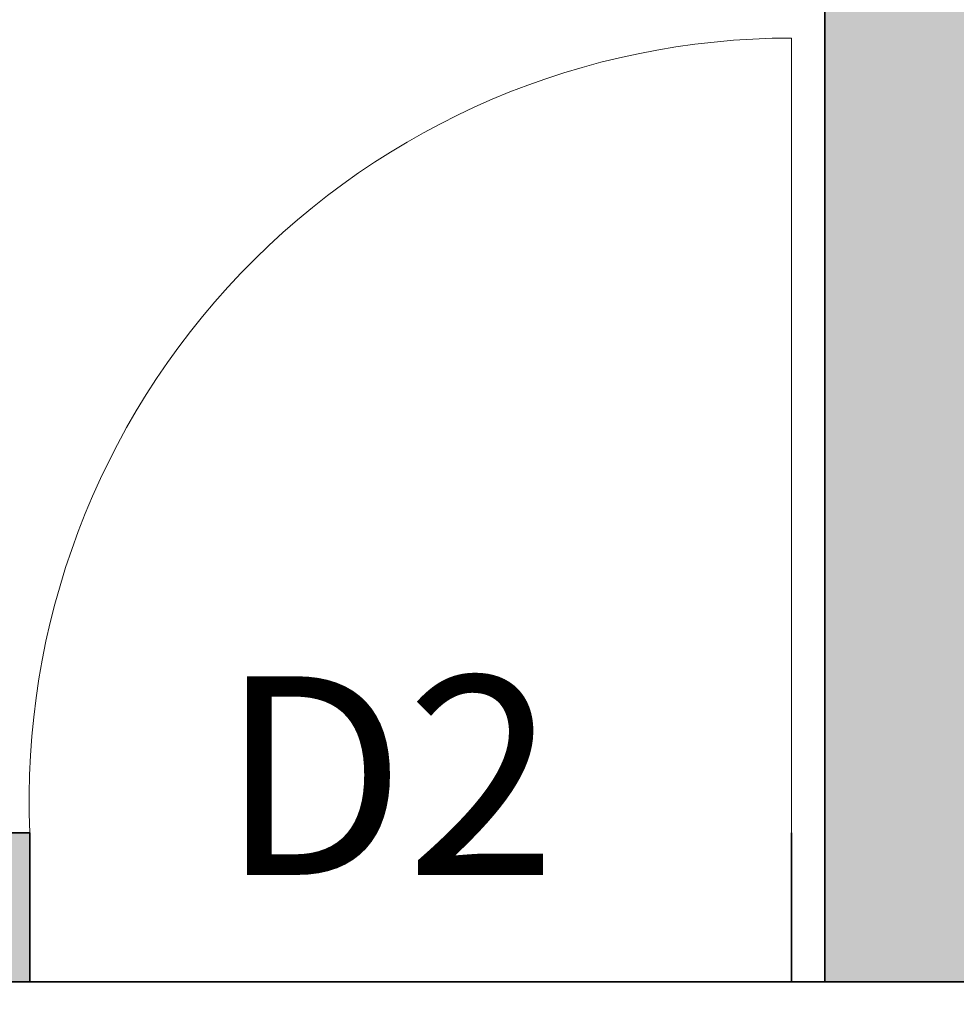
# Model space of a CAD drawing. Units: inches. Extents: x -9 to 505, y -680 to 48.
# Tile 13 of 17: x 96 to 124, y -169 to -139. Entities that reach past the tile are written whole.
import ezdxf

# ---------------------------------------------------------------- set-up
doc = ezdxf.new("R2010")
doc.units = ezdxf.units.IN
doc.header["$MEASUREMENT"] = 0
for name, color, linetype, lineweight in [('A-ANNO-TEXT', 7, 'Continuous', 18), ('A-DOOR', 3, 'Continuous', 18), ('A-WALL', 7, 'Continuous', 35), ('A-WALL-PATT', 251, 'Continuous', 13)]:
    doc.layers.add(name, color=color, linetype=linetype, lineweight=lineweight)
doc.styles.get("Standard").update_dxf_attribs({"font": 'arial.ttf'})

msp = doc.modelspace()

# ---------------------------------------------------------------- hatches: boundary and pattern name
at = {"layer": 'A-WALL-PATT'}
h = msp.add_hatch(color=256, dxfattribs=at)
h.dxf.hatch_style = 1
h.paths.add_polyline_path([(101.641, 11.499), (48.264, 11.499), (48.264, 2.499), (72.264, 2.499), (72.264, -21.248), (81.264, -21.248), (81.264, 2.499), (101.641, 2.499)])
h.paths.add_polyline_path([(36.264, 2.499), (27.264, 2.499), (27.264, -6.918), (36.264, -6.918)])
h.paths.add_polyline_path([(81.264, -57.248), (72.264, -57.248), (72.264, -75.501), (81.264, -75.501)])
h.paths.add_polyline_path([(162.764, 11.499), (137.641, 11.499), (137.641, 2.499), (162.764, 2.499)])
h.paths.add_polyline_path([(179.264, 2.499), (174.764, 2.499), (174.764, -75.501), (179.264, -75.501), (179.264, -54.501), (229.514, -54.501), (229.514, -45.501), (179.264, -45.501)])
h.paths.add_polyline_path([(382.256, -45.501), (332.264, -45.501), (332.264, 2.499), (327.764, 2.499), (327.764, -45.501), (277.514, -45.501), (277.514, -54.501), (327.764, -54.501), (327.764, -111.501), (332.264, -111.501), (332.264, -54.501), (382.256, -54.501)])
h.paths.add_polyline_path([(332.264, -128.001), (327.764, -128.001), (327.764, -207.001), (332.264, -207.001)])
h.paths.add_polyline_path([(124.764, -111.501), (36.264, -111.501), (36.264, -116.001), (120.264, -116.001), (120.264, -168.501), (179.264, -168.501), (179.264, -164.001), (124.764, -164.001)])
h.paths.add_polyline_path([(96.264, -164.001), (36.264, -164.001), (36.264, -152.001), (27.264, -152.001), (27.264, -208.879), (36.264, -208.879), (36.264, -168.501), (96.264, -168.501)])
h.paths.add_polyline_path([(36.264, -244.879), (27.264, -244.879), (27.264, -287.001), (36.264, -287.001)])
h.paths.add_polyline_path([(179.264, -204.501), (174.764, -204.501), (174.764, -287.001), (179.264, -287.001)])
h.paths.add_polyline_path([(257.264, -296.001), (248.264, -296.001), (248.264, -446.001), (269.264, -446.001), (269.264, -437.001), (257.264, -437.001)])
h.paths.add_polyline_path([(90.264, -296.001), (81.264, -296.001), (81.264, -348.67), (90.264, -348.67)])
h.paths.add_polyline_path([(90.264, -384.67), (81.264, -384.67), (81.264, -416.001), (90.264, -416.001)])
h.paths.add_polyline_path([(170.264, -452.001), (36.264, -452.001), (36.264, -456.501), (165.764, -456.501), (165.764, -504.501), (165.133, -504.501), (165.133, -509.001), (170.264, -509.001)])
h.paths.add_polyline_path([(141.764, -504.501), (36.264, -504.501), (36.264, -492.501), (27.264, -492.501), (27.264, -565.959), (36.264, -565.959), (36.264, -509.001), (141.764, -509.001)])
h.paths.add_polyline_path([(36.264, -601.959), (27.264, -601.959), (27.264, -658.501), (36.264, -658.501)])
h.paths.add_polyline_path([(170.264, -670.501), (170.264, -634.501), (222.764, -634.501), (222.764, -625.501), (165.764, -625.501), (165.764, -670.501), (36.264, -670.501), (36.264, -679.501), (170.264, -679.501)])
h.paths.add_polyline_path([(332.264, -616.501), (433.894, -616.501), (433.894, -612.001), (332.264, -612.001), (332.264, -610.563), (327.764, -610.563), (327.764, -625.501), (270.764, -625.501), (270.764, -634.501), (327.764, -634.501), (327.764, -658.501), (332.264, -658.501)])
h.paths.add_polyline_path([(459.764, -670.501), (336.764, -670.501), (336.764, -679.501), (459.764, -679.501)])
h.paths.add_polyline_path([(468.764, -545.737), (459.764, -545.737), (459.764, -612.001), (457.894, -612.001), (457.894, -616.501), (459.764, -616.501), (459.764, -658.501), (468.764, -658.501)])
h.paths.add_polyline_path([(332.264, -446.001), (327.764, -446.001), (327.764, -574.563), (332.264, -574.563)])
h.paths.add_polyline_path([(327.764, -437.001), (305.264, -437.001), (305.264, -446.001), (327.764, -446.001)])
h.paths.add_polyline_path([(459.764, -437.001), (348.764, -437.001), (348.764, -446.001), (459.764, -446.001)])
h.paths.add_polyline_path([(468.764, -458.001), (459.764, -458.001), (459.764, -509.737), (468.764, -509.737)])
h.paths.add_polyline_path([(468.764, -365.001), (459.764, -365.001), (459.764, -437.001), (468.764, -437.001)])
h.paths.add_polyline_path([(468.764, -299.601), (459.764, -299.601), (459.764, -344.001), (468.764, -344.001)])
h.paths.add_polyline_path([(468.764, -184.739), (459.764, -184.739), (459.764, -231.001), (401.264, -231.001), (401.264, -235.501), (459.764, -235.501), (459.764, -275.601), (468.764, -275.601)])
h.paths.add_polyline_path([(390.764, -356.001), (342.764, -356.001), (342.764, -365.001), (390.764, -365.001)])
h.paths.add_polyline_path([(459.764, -356.001), (405.764, -356.001), (405.764, -365.001), (459.764, -365.001)])
h.paths.add_polyline_path([(405.764, -296.001), (396.764, -296.001), (396.764, -356.001), (405.764, -356.001)])
h.paths.add_polyline_path([(336.764, -296.001), (327.764, -296.001), (327.764, -356.001), (336.764, -356.001)])
h.paths.add_polyline_path([(468.764, -9.501), (459.764, -9.501), (459.764, -45.501), (418.256, -45.501), (418.256, -54.501), (468.764, -54.501)])
h.paths.add_polyline_path([(468.764, -54.501), (459.764, -54.501), (459.764, -111.501), (468.764, -111.501)])
h.paths.add_polyline_path([(468.764, -128.001), (459.764, -128.001), (459.764, -148.739), (468.764, -148.739)])

# ---------------------------------------------------------------- linework, layer by layer
at = {"layer": 'A-DOOR'}
msp.add_line((119.264, -163.993), (119.264, -139.993), dxfattribs=at)
msp.add_arc((119.264, -163.015), 23.021, 90, 182.4556, dxfattribs=at)
at = {"layer": 'A-WALL'}
for p, q in [((120.264, -116.001), (120.264, -168.501)), ((36.264, -164.001), (96.264, -164.001)), ((96.264, -164.001), (96.264, -168.501)), ((119.264, -163.993), (119.264, -168.501)), ((36.264, -168.501), (179.264, -168.501))]:
    msp.add_line(p, q, dxfattribs=at)

# ---------------------------------------------------------------- texts
at = {"layer": 'A-ANNO-TEXT', "insert": (101.988, -159.269), "char_height": 6, "attachment_point": 1}
msp.add_mtext('D2', dxfattribs=at)

doc.saveas('drawing.dxf')
